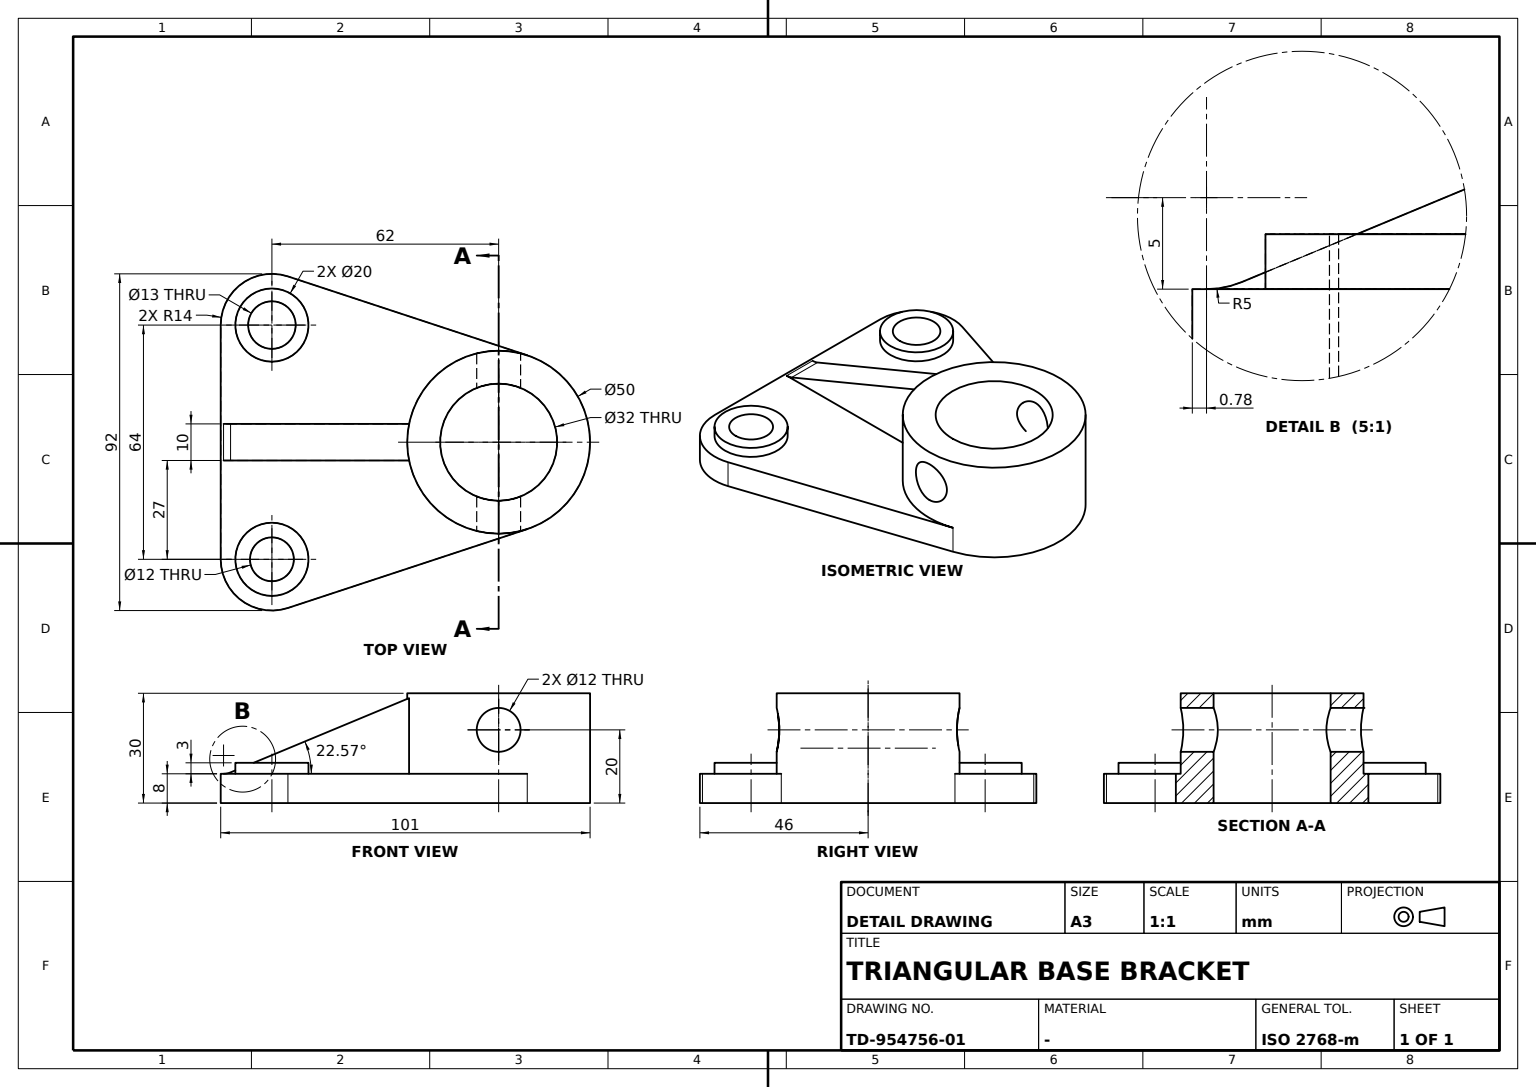
CATIA V5 part; units mm, degrees
sketch "Sketch1" plane through (0, 0, 0) normal (0, 0, 1) x (1, 0, 0)
  arc A0 (23.7454, 7.8202) -> (-23.7454, 7.8202) centre (0, 0) ccw
  arc A1 (-45.2974, -57.6207) -> (-32, -76) centre (-32, -62) ccw
  point P0 (-32, -62)
  arc A2 (32, -76) -> (45.2974, -57.6207) centre (32, -62) ccw
  point P1 (32, -62)
  line L0 (-23.7454, 7.8202) -> (-45.2974, -57.6207)
  line L1 (23.7454, 7.8202) -> (45.2974, -57.6207)
  line L2 (-32, -76) -> (32, -76)
  dimension "radius A0" = 25
  dimension "radius A2" = 14
  dimension "radius A1" = 14
  dimension "distance P0 P1" = 64
  dimension "distance x axis P1" = 62
  constraint symmetry P0 P1 y-axis
  constraint tangency L0 A0
  constraint tangency L0 A1
  constraint tangency L1 A0
  constraint tangency L1 A2
  constraint tangency L2 A1
  constraint tangency L2 A2
extrude "Pad1" add sketch "Sketch1" along normal blind 8
sketch "Sketch2" plane through (0, 0, 8) normal (0, 0, 1) x (1, 0, 0)
  circle A0 centre (0, 0) radius 25
  circle A1 centre (0, 0) radius 16
  dimension "radius A0" = 25
  dimension "radius A1" = 16
extrude "Pad2" add sketch "Sketch2" along normal blind 22
sketch "Pocket1 profile" plane through (0, 0, 8) normal (0, 0, 1) x (1, 0, 0)
  circle A0 centre (0, 0) radius 16
extrude "Pocket1" cut sketch "Pocket1 profile" against normal blind 22
sketch "Sketch3" plane through (0, 0, 0) normal (1, 0, 0) x (0, 1, 0)
  line L0 (-76, 7.2622) -> (-22.618, 29.4517)
  point P0 (-76, 7.2622)
  line L1 (-76, 0) -> (-76, 8) construction
  constraint coincidence P0 L1
rib "Stiffener1" sketch "Sketch3" thickness 10 sides both
sketch "Sketch4" plane through (0, 0, 8) normal (0, 0, 1) x (1, 0, 0)
  circle A0 centre (-32, -62) radius 10
  point P0 (-32, -62)
  circle A1 centre (32, -62) radius 10
  point P1 (32, -62)
  circle A2 centre (32, -62) radius 6
  circle A3 centre (-32, -62) radius 6.5
  dimension "distance x axis P0" = 62
  dimension "radius A0" = 10
  dimension "radius A1" = 10
  dimension "distance P0 P1" = 64
  dimension "radius A2" = 6
  dimension "radius A3" = 6.5
  constraint symmetry P0 P1 y-axis
extrude "Pad3" add sketch "Sketch4" along normal blind 3
sketch "Pocket2 profile" plane through (0, 0, 8) normal (0, 0, 1) x (1, 0, 0)
  circle A0 centre (32, -62) radius 6
extrude "Pocket2" cut sketch "Pocket2 profile" against normal up to next
sketch "Pocket3 profile" plane through (0, 0, 8) normal (0, 0, 1) x (1, 0, 0)
  circle A0 centre (-32, -62) radius 6.5
extrude "Pocket3" cut sketch "Pocket3 profile" against normal through all
sketch "Sketch5" plane through (0, 0, 0) normal (1, 0, 0) x (0, 1, 0)
  circle A0 centre (0, 20) radius 6
  point P0 (0, 20)
  line L0 (-16, 30) -> (16, 30) construction
  dimension "radius A0" = 6
  dimension "distance L0 P0" = 10
  constraint coincidence P0 y-axis
extrude "Pocket4" cut sketch "Sketch5" along normal through all
sketch "Sketch6" plane through (0, 0, 0) normal (1, 0, 0) x (0, 1, 0)
  circle A0 centre (0, 20) radius 6
  point P0 (0, 20)
  line L0 (-25, 30) -> (25, 30) construction
  dimension "radius A0" = 6
  dimension "distance L0 P0" = 10
extrude "Pocket5" cut sketch "Sketch6" against normal through all
fillet "Fillet1" radius 5 1 edges at (0, -74.2251, 8)
